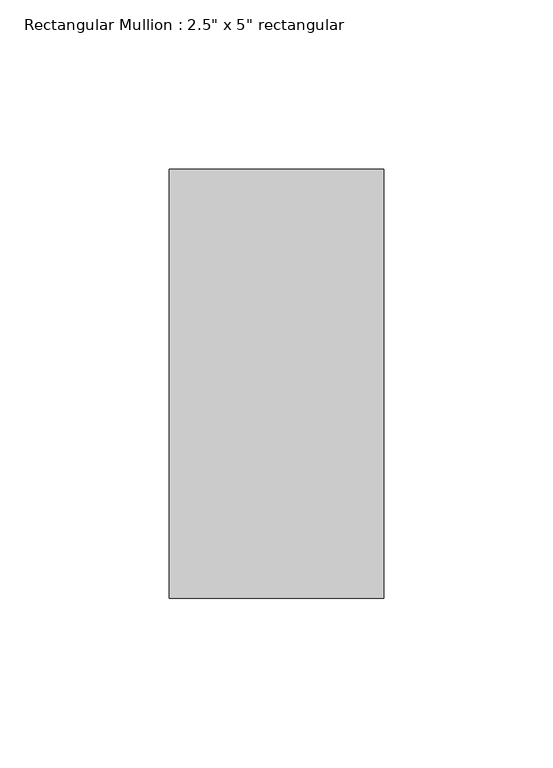
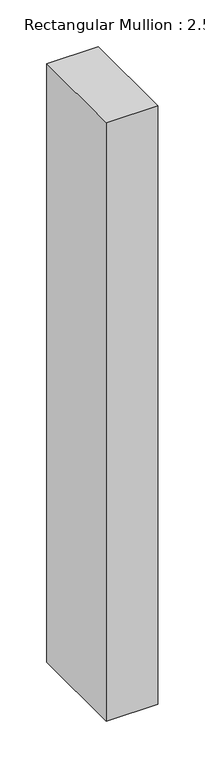
"""IFC4 building model written with IfcOpenShell, lengths in millimetres: member geometry."""

from ifc_helpers import new_model, si_unit, frame, origin, place, context, project, spatial, polyline, outline, extrude, source, transform, mapped, element, save


def member_a1032ffb(model_context):
    return source(origin(), model_context, "Body", "SweptSolid", [
        extrude(outline(polyline([(0.0, 63.5), (0.0, -63.5), (-63.5, -63.5), (-63.5, 63.5), (0.0, 63.5)])), frame((0.0, 0.0, -780.2809615), z_axis=(0.0, 0.0, 1.0), x_axis=(1.0, 0.0, 0.0)), (0.0, 0.0, 1.0), 780.2809615),
    ])


if __name__ == "__main__":
    model = new_model("IFC4")
    model_context = context("Model", 3, world=origin())
    ifc_project = project(units=[si_unit("LENGTHUNIT", "METRE", prefix="MILLI")], contexts=[model_context])
    site = spatial("IfcSite", under=ifc_project)
    building = spatial("IfcBuilding", under=site)
    placement = place(None, origin())
    member_shape = member_a1032ffb(model_context)
    element("IfcMember", 1, ObjectType="Rectangular Mullion : 2.5\" x 5\" rectangular", at=placement, inside=building, context=model_context, shape_type="MappedRepresentation", body=[
        mapped(member_shape, transform((0.0, 0.0, 0.0), x_axis=(1.0, 0.0, 0.0), y_axis=(0.0, 1.0, 0.0), z_axis=(0.0, 0.0, 1.0))),
    ])
    save(model, "model.ifc")

# Revit data of these elements
# Type "Rectangular Mullion : 2.5\" x 5\" rectangular"
#   built-in parameter 1007304 = 0.416667 (stored number, unit not read)
#   built-in parameter 1007301 = 0.104167 (stored number, unit not read)
#   built-in parameter 1007300 = 0.104167 (stored number, unit not read)
# Element 1 (IfcMember, "Rectangular Mullion : 2.5\" x 5\" rectangular")
#   Materials on its faces: "Aluminum"
# Materials
#   "Aluminum": class "Metal", colour RGB 247 247 247, transparency 0, Description = "Aluminum 6061", Cost = 0
